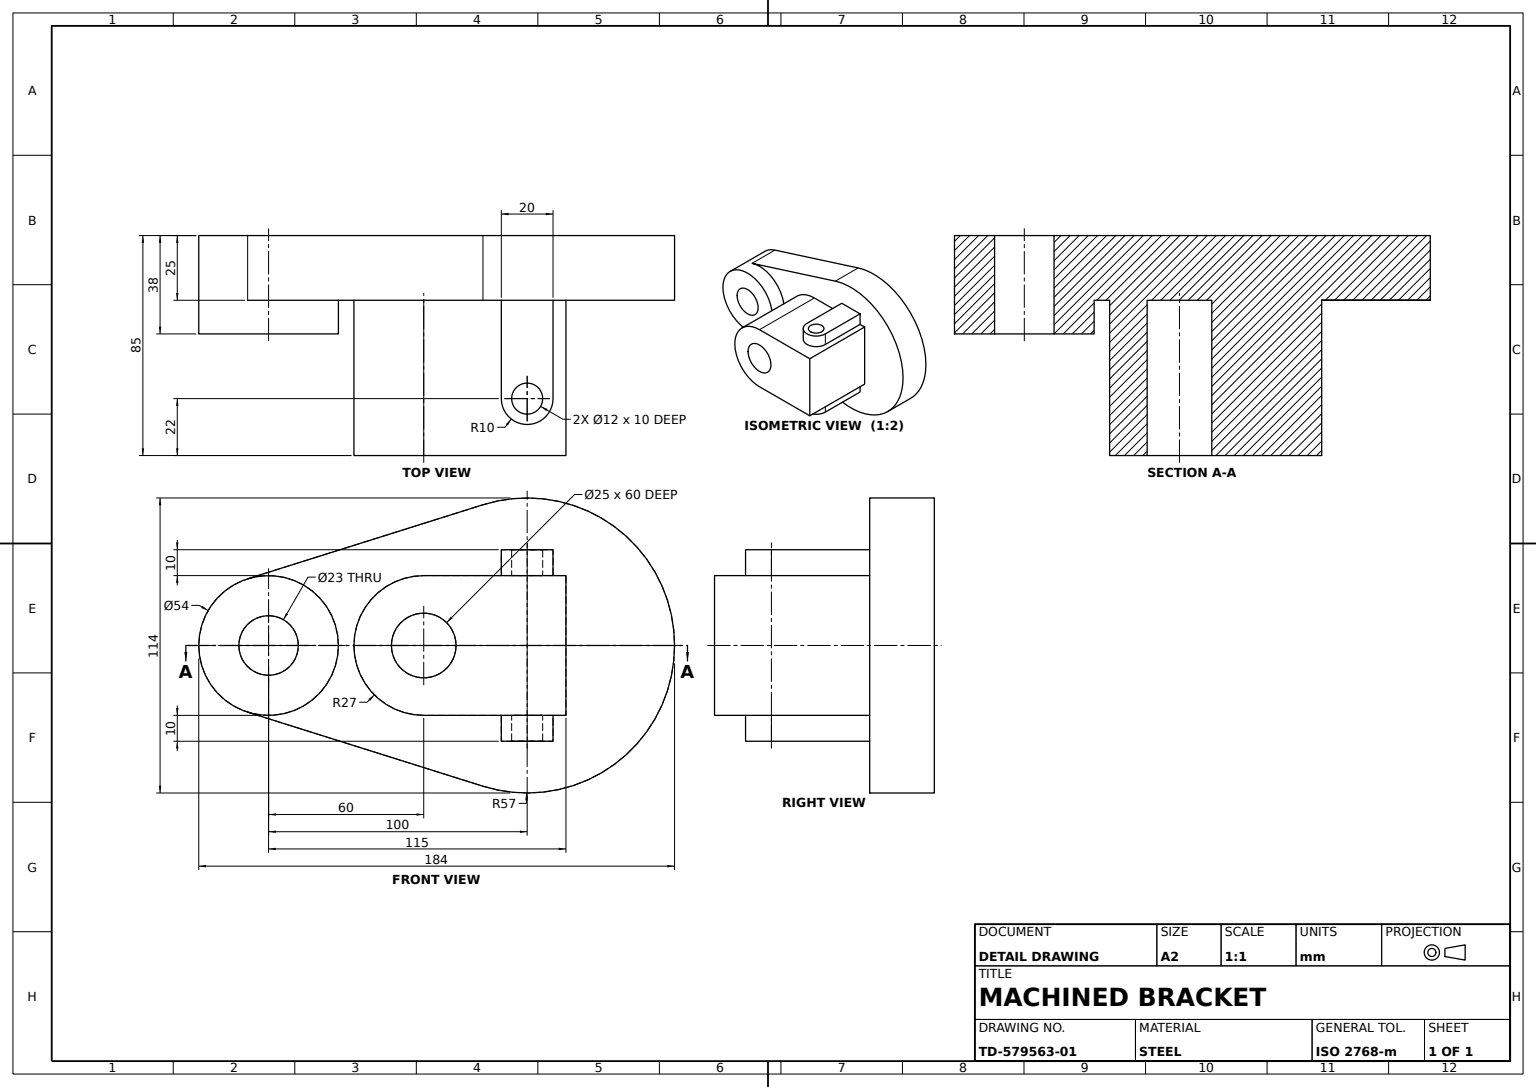
from build123d import *

# Parameters (mm, degrees)
PIVOT_BOSS_SKETCH_R   = 27
PIVOT_BOSS_SKETCH_R_2 = 11.5
PIVOT_BOSS_DEPTH      = 38
MOUNTING_PLATE_DEPTH  = 25
ARM_BLOCK_DEPTH       = 60
PIVOT_BORE_SKETCH_R   = 12.5
PIVOT_BORE_25_DEPTH   = 60
CLAMP_TAB_SKETCH_R    = 6
CLAMP_TAB_DEPTH       = 10


with BuildPart() as part:
    # Pivot Boss Sketch → Pivot Boss (new body)
    with BuildSketch(Plane.XY):
        Circle(PIVOT_BOSS_SKETCH_R)
        Circle(PIVOT_BOSS_SKETCH_R_2, mode=Mode.SUBTRACT)
    extrude(amount=PIVOT_BOSS_DEPTH)

    # Mounting Plate Sketch → Mounting Plate (add)
    with BuildSketch(Plane.XY):
        with BuildLine():
            Line((-8.1, 25.756358438), (82.9, 54.374534481))
            ThreePointArc((82.9, 54.374534481), (157, 0), (82.9, -54.374534481))
            Line((82.9, -54.374534481), (-8.1, -25.756358438))
            ThreePointArc((-8.1, -25.756358438), (27, 0), (-8.1, 25.756358438))
        make_face()
    extrude(amount=MOUNTING_PLATE_DEPTH)

    # Arm Block Sketch → Arm Block (add)
    with BuildSketch(Plane.XY.offset(25)):
        with BuildLine():
            Line((60, 27), (115, 27))
            Line((115, 27), (115, -27))
            Line((115, -27), (60, -27))
            ThreePointArc((60, -27), (33, 0), (60, 27))
        make_face()
    extrude(amount=ARM_BLOCK_DEPTH)

    # Pivot Bore Sketch → Pivot Bore Ø25 (cut)
    with BuildSketch(Plane.XY.offset(85)):
        with Locations((60, 0)):
            Circle(PIVOT_BORE_SKETCH_R)
    extrude(amount=-PIVOT_BORE_25_DEPTH, mode=Mode.SUBTRACT)

    # Clamp Tab Sketch → Clamp Tab (add)
    with BuildSketch(Plane.XZ.offset(27)):
        with BuildLine():
            Line((90, 63), (90, 25))
            Line((90, 25), (110, 25))
            Line((110, 25), (110, 63))
            ThreePointArc((110, 63), (100, 73), (90, 63))
        make_face()
        with Locations(Location((100, 63, 0), (0, 0, 270))):
            Circle(CLAMP_TAB_SKETCH_R, mode=Mode.SUBTRACT)
    clamp_tab = extrude(amount=CLAMP_TAB_DEPTH)

    # Clamp Tab Mirror: Clamp Tab across plane
    add(clamp_tab.mirror(Plane.ZX))


solid = part.part
